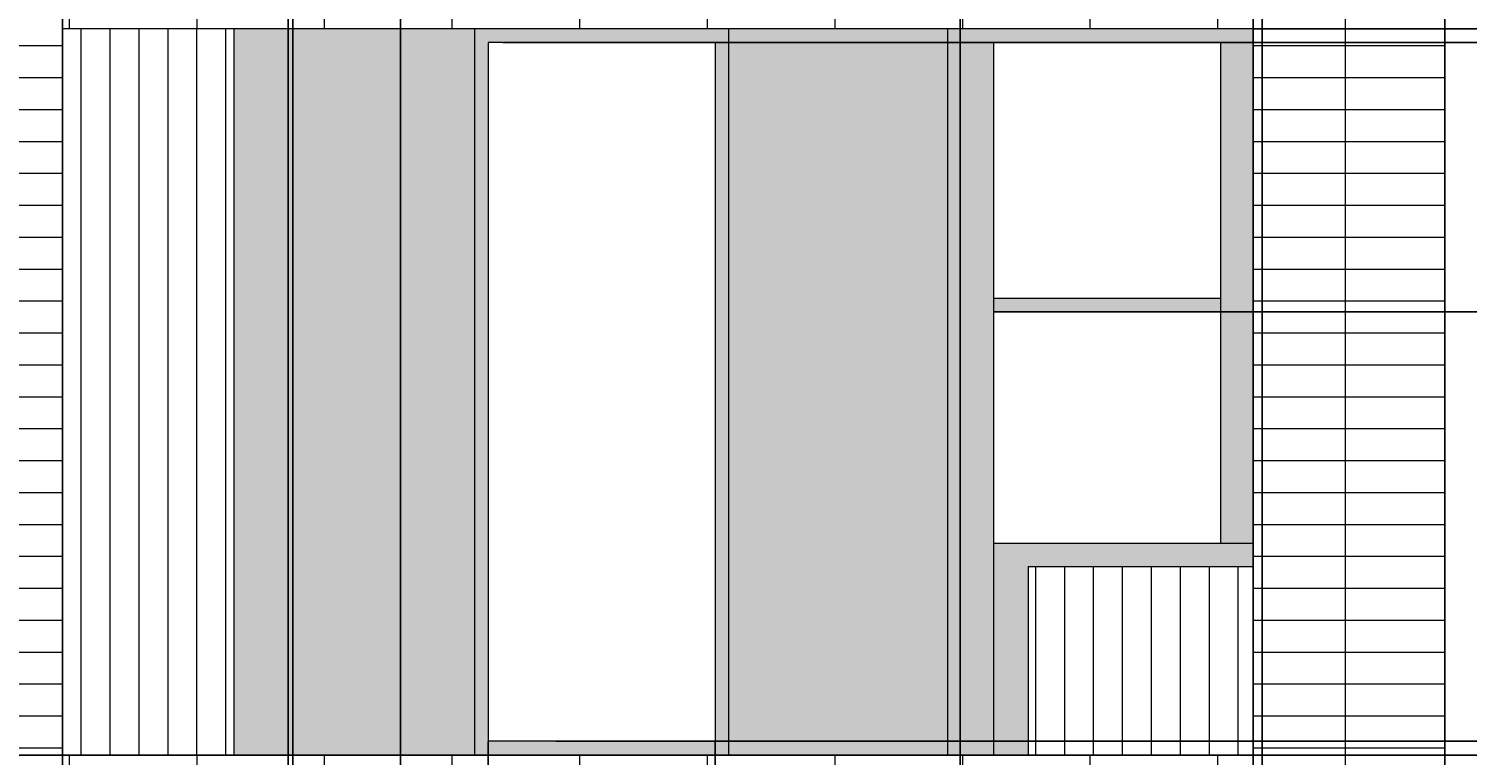
# Model space of a CAD drawing. Units: inches. Extents: x 241 to 943, y 109 to 1396.
# Tile 16 of 34: x 613 to 824, y 735 to 842. Entities that reach past the tile are written whole.
import ezdxf

# ---------------------------------------------------------------- set-up
doc = ezdxf.new("R2010")
doc.units = ezdxf.units.IN
doc.header["$MEASUREMENT"] = 0
for name, color, linetype, lineweight in [('A-ANNO-DIMS', 2, 'Continuous', 18), ('A-ELEV', 7, 'Continuous', 25), ('A-ELEV-SHAD', 9, 'Continuous', 13), ('A-GLAZ', 4, 'Continuous', 18), ('A-GLAZ-PATT', 18, 'Continuous', 13), ('A-WALL-PATT', 8, 'Continuous', 13)]:
    doc.layers.add(name, color=color, linetype=linetype, lineweight=lineweight)
doc.styles.get("Standard").update_dxf_attribs({"font": 'arial.ttf'})
doc.dimstyles.get("Standard").update_dxf_attribs({"dimtxt": 1.4375, "dimasz": 0.18, "dimexe": 0.18, "dimexo": 0.0625, "dimgap": 0.09, "dimtad": 0, "dimtih": 1, "dimtoh": 1, "dimdec": 4, "dimzin": 0, "dimdsep": 46, "dimlunit": 4, "dimtxsty": 'Standard', "dimcen": 0.09, "dimadec": 0, "dimazin": 0, "dimtfac": 1, "dimtdec": 4, "dimtofl": 0, "dimtmove": 0, "dimatfit": 3, "dimfxl": 1, "dimtolj": 1, "dimtzin": 0, "dimarcsym": 0})

# ---------------------------------------------------------------- blocks, each defined once
blk = doc.blocks.new('*D6')
at = {"layer": 'A-ANNO-DIMS', "color": 0, "lineweight": -2, "transparency": 16777216}
for p, q in [((820.84, 232.89), (820.84, 1395.05)), ((881.67, 232.89), (881.67, 1395.05)), ((821.02, 1394.87), (848.73, 1394.87)), ((881.49, 1394.87), (853.77, 1394.87))]:
    blk.add_line(p, q, dxfattribs=at)
at = {"layer": 'A-ANNO-DIMS', "color": 0, "transparency": 16777216}
for points in [[(821.02, 1394.9), (821.02, 1394.84), (820.84, 1394.87)], [(881.49, 1394.9), (881.49, 1394.84), (881.67, 1394.87)]]:
    blk.add_solid(points, dxfattribs=at)
at = {"layer": 'Defpoints', "color": 0, "transparency": 16777216}
for p in [(881.67, 1394.87), (820.84, 232.83), (881.67, 232.83)]:
    blk.add_point(p, dxfattribs=at)
at = {"layer": 'A-ANNO-DIMS', "color": 0, "transparency": 16777216, "insert": (851.25, 1394.87), "char_height": 1.438, "attachment_point": 5}
blk.add_mtext('\\A1;60.83', dxfattribs=at)
blk = doc.blocks.new('*D12')
at = {"layer": 'A-ANNO-DIMS', "color": 0, "lineweight": -2, "transparency": 16777216}
for p, q in [((530.23, 384.24), (530.23, 1395.05)), ((650.91, 384.24), (650.91, 1395.05)), ((530.41, 1394.87), (587.56, 1394.87)), ((650.73, 1394.87), (593.58, 1394.87))]:
    blk.add_line(p, q, dxfattribs=at)
at = {"layer": 'A-ANNO-DIMS', "color": 0, "transparency": 16777216}
for points in [[(530.41, 1394.9), (530.41, 1394.84), (530.23, 1394.87)], [(650.73, 1394.9), (650.73, 1394.84), (650.91, 1394.87)]]:
    blk.add_solid(points, dxfattribs=at)
at = {"layer": 'Defpoints', "color": 0, "transparency": 16777216}
for p in [(650.91, 1394.87), (530.23, 384.18), (650.91, 384.18)]:
    blk.add_point(p, dxfattribs=at)
at = {"layer": 'A-ANNO-DIMS', "color": 0, "transparency": 16777216, "insert": (590.57, 1394.87), "char_height": 1.438, "attachment_point": 5}
blk.add_mtext('\\A1;120.68', dxfattribs=at)
blk = doc.blocks.new('*D13')
at = {"layer": 'A-ANNO-DIMS', "color": 0, "lineweight": -2, "transparency": 16777216}
for p, q in [((650.91, 384.24), (650.91, 1395.05)), ((667.39, 290.06), (667.39, 1395.05)), ((651.09, 1394.87), (656.14, 1394.87)), ((667.21, 1394.87), (662.16, 1394.87))]:
    blk.add_line(p, q, dxfattribs=at)
at = {"layer": 'A-ANNO-DIMS', "color": 0, "transparency": 16777216}
for points in [[(651.09, 1394.9), (651.09, 1394.84), (650.91, 1394.87)], [(667.21, 1394.9), (667.21, 1394.84), (667.39, 1394.87)]]:
    blk.add_solid(points, dxfattribs=at)
at = {"layer": 'Defpoints', "color": 0, "transparency": 16777216}
for p in [(667.39, 1394.87), (650.91, 384.18), (667.39, 290)]:
    blk.add_point(p, dxfattribs=at)
at = {"layer": 'A-ANNO-DIMS', "color": 0, "transparency": 16777216, "insert": (659.15, 1394.87), "char_height": 1.438, "attachment_point": 5}
blk.add_mtext('\\A1;16.486', dxfattribs=at)
blk = doc.blocks.new('*D14')
at = {"layer": 'A-ANNO-DIMS', "color": 0, "lineweight": -2, "transparency": 16777216}
for p, q in [((667.39, 290.06), (667.39, 1395.05)), ((794.03, 290.06), (794.03, 1395.05)), ((667.57, 1394.87), (727.7, 1394.87)), ((793.85, 1394.87), (733.72, 1394.87))]:
    blk.add_line(p, q, dxfattribs=at)
at = {"layer": 'A-ANNO-DIMS', "color": 0, "transparency": 16777216}
for points in [[(667.57, 1394.9), (667.57, 1394.84), (667.39, 1394.87)], [(793.85, 1394.9), (793.85, 1394.84), (794.03, 1394.87)]]:
    blk.add_solid(points, dxfattribs=at)
at = {"layer": 'Defpoints', "color": 0, "transparency": 16777216}
for p in [(794.03, 1394.87), (667.39, 290), (794.03, 290)]:
    blk.add_point(p, dxfattribs=at)
at = {"layer": 'A-ANNO-DIMS', "color": 0, "transparency": 16777216, "insert": (730.71, 1394.87), "char_height": 1.438, "attachment_point": 5}
blk.add_mtext('\\A1;126.63', dxfattribs=at)
blk = doc.blocks.new('*D15')
at = {"layer": 'A-ANNO-DIMS', "color": 0, "lineweight": -2, "transparency": 16777216}
for p, q in [((794.03, 290.06), (794.03, 1395.05)), ((820.84, 232.89), (820.84, 1395.05)), ((794.21, 1394.87), (805.04, 1394.87)), ((820.66, 1394.87), (809.82, 1394.87))]:
    blk.add_line(p, q, dxfattribs=at)
at = {"layer": 'A-ANNO-DIMS', "color": 0, "transparency": 16777216}
for points in [[(794.21, 1394.9), (794.21, 1394.84), (794.03, 1394.87)], [(820.66, 1394.9), (820.66, 1394.84), (820.84, 1394.87)]]:
    blk.add_solid(points, dxfattribs=at)
at = {"layer": 'Defpoints', "color": 0, "transparency": 16777216}
for p in [(820.84, 1394.87), (794.03, 290), (820.84, 232.83)]:
    blk.add_point(p, dxfattribs=at)
at = {"layer": 'A-ANNO-DIMS', "color": 0, "transparency": 16777216, "insert": (807.43, 1394.87), "char_height": 1.438, "attachment_point": 5}
blk.add_mtext('\\A1;26.81', dxfattribs=at)
blk = doc.blocks.new('*D47')
at = {"layer": 'A-ANNO-DIMS', "color": 0, "lineweight": -2, "transparency": 16777216}
for p, q in [((792.75, 841.54), (940.6, 841.54)), ((940.42, 841.36), (940.42, 789.02)), ((940.42, 735.03), (940.42, 787.37)), ((792.75, 734.85), (940.6, 734.85))]:
    blk.add_line(p, q, dxfattribs=at)
at = {"layer": 'A-ANNO-DIMS', "color": 0, "transparency": 16777216}
for points in [[(940.39, 841.36), (940.45, 841.36), (940.42, 841.54)], [(940.39, 735.03), (940.45, 735.03), (940.42, 734.85)]]:
    blk.add_solid(points, dxfattribs=at)
at = {"layer": 'Defpoints', "color": 0, "transparency": 16777216}
for p in [(792.69, 841.54), (940.42, 841.54), (792.69, 734.85)]:
    blk.add_point(p, dxfattribs=at)
at = {"layer": 'A-ANNO-DIMS', "color": 0, "transparency": 16777216, "insert": (940.42, 788.2), "char_height": 1.438, "attachment_point": 5}
blk.add_mtext('\\A1;106.68', dxfattribs=at)
blk = doc.blocks.new('*D63')
at = {"layer": 'A-ANNO-DIMS', "color": 0, "lineweight": -2, "transparency": 16777216}
for p, q in [((651.6, 568.89), (651.6, 1395.05)), ((792.69, 568.89), (792.69, 1395.05)), ((651.78, 1394.87), (719.84, 1394.87)), ((792.51, 1394.87), (724.45, 1394.87))]:
    blk.add_line(p, q, dxfattribs=at)
at = {"layer": 'A-ANNO-DIMS', "color": 0, "transparency": 16777216}
for points in [[(651.78, 1394.9), (651.78, 1394.84), (651.6, 1394.87)], [(792.51, 1394.9), (792.51, 1394.84), (792.69, 1394.87)]]:
    blk.add_solid(points, dxfattribs=at)
at = {"layer": 'Defpoints', "color": 0, "transparency": 16777216}
for p in [(792.69, 1394.87), (651.6, 568.83), (792.69, 568.83)]:
    blk.add_point(p, dxfattribs=at)
at = {"layer": 'A-ANNO-DIMS', "color": 0, "transparency": 16777216, "insert": (722.14, 1394.87), "char_height": 1.438, "attachment_point": 5}
blk.add_mtext('\\A1;141.1', dxfattribs=at)
blk = doc.blocks.new('*D64')
at = {"layer": 'A-ANNO-DIMS', "color": 0, "lineweight": -2, "transparency": 16777216}
for p, q in [((792.69, 568.89), (792.69, 1395.05)), ((820.84, 568.89), (820.84, 1395.05)), ((792.87, 1394.87), (803.68, 1394.87)), ((820.66, 1394.87), (809.85, 1394.87))]:
    blk.add_line(p, q, dxfattribs=at)
at = {"layer": 'A-ANNO-DIMS', "color": 0, "transparency": 16777216}
for points in [[(792.87, 1394.9), (792.87, 1394.84), (792.69, 1394.87)], [(820.66, 1394.9), (820.66, 1394.84), (820.84, 1394.87)]]:
    blk.add_solid(points, dxfattribs=at)
at = {"layer": 'Defpoints', "color": 0, "transparency": 16777216}
for p in [(820.84, 1394.87), (792.69, 568.83), (820.84, 568.83)]:
    blk.add_point(p, dxfattribs=at)
at = {"layer": 'A-ANNO-DIMS', "color": 0, "transparency": 16777216, "insert": (806.76, 1394.87), "char_height": 1.438, "attachment_point": 5}
blk.add_mtext('\\A1;28.146', dxfattribs=at)
blk = doc.blocks.new('*D66')
at = {"layer": 'A-ANNO-DIMS', "color": 0, "lineweight": -2, "transparency": 16777216}
for p, q in [((617.76, 702.85), (617.76, 1395.05)), ((749.63, 702.85), (749.63, 1395.05)), ((617.94, 1394.87), (680.69, 1394.87)), ((749.45, 1394.87), (686.7, 1394.87))]:
    blk.add_line(p, q, dxfattribs=at)
at = {"layer": 'A-ANNO-DIMS', "color": 0, "transparency": 16777216}
for points in [[(617.94, 1394.9), (617.94, 1394.84), (617.76, 1394.87)], [(749.45, 1394.9), (749.45, 1394.84), (749.63, 1394.87)]]:
    blk.add_solid(points, dxfattribs=at)
at = {"layer": 'Defpoints', "color": 0, "transparency": 16777216}
for p in [(749.63, 1394.87), (617.76, 702.79), (749.63, 702.79)]:
    blk.add_point(p, dxfattribs=at)
at = {"layer": 'A-ANNO-DIMS', "color": 0, "transparency": 16777216, "insert": (683.7, 1394.87), "char_height": 1.438, "attachment_point": 5}
blk.add_mtext('\\A1;131.87', dxfattribs=at)
blk = doc.blocks.new('*D82')
at = {"layer": 'A-ANNO-DIMS', "color": 0, "lineweight": -2, "transparency": 16777216}
for p, q in [((565.2, 568.89), (565.2, 1395.05)), ((651.6, 568.89), (651.6, 1395.05)), ((565.38, 1394.87), (605.89, 1394.87)), ((651.42, 1394.87), (610.91, 1394.87))]:
    blk.add_line(p, q, dxfattribs=at)
at = {"layer": 'A-ANNO-DIMS', "color": 0, "transparency": 16777216}
for points in [[(565.38, 1394.9), (565.38, 1394.84), (565.2, 1394.87)], [(651.42, 1394.9), (651.42, 1394.84), (651.6, 1394.87)]]:
    blk.add_solid(points, dxfattribs=at)
at = {"layer": 'Defpoints', "color": 0, "transparency": 16777216}
for p in [(651.6, 1394.87), (565.2, 568.83), (651.6, 568.83)]:
    blk.add_point(p, dxfattribs=at)
at = {"layer": 'A-ANNO-DIMS', "color": 0, "transparency": 16777216, "insert": (608.4, 1394.87), "char_height": 1.438, "attachment_point": 5}
blk.add_mtext('\\A1;86.40', dxfattribs=at)
blk = doc.blocks.new('*D83')
at = {"layer": 'A-ANNO-DIMS', "color": 0, "lineweight": -2, "transparency": 16777216}
for p, q in [((592.95, 700.85), (592.95, 1395.05)), ((617.76, 702.85), (617.76, 1395.05)), ((593.13, 1394.87), (602.27, 1394.87)), ((617.58, 1394.87), (608.45, 1394.87))]:
    blk.add_line(p, q, dxfattribs=at)
at = {"layer": 'A-ANNO-DIMS', "color": 0, "transparency": 16777216}
for points in [[(593.13, 1394.9), (593.13, 1394.84), (592.95, 1394.87)], [(617.58, 1394.9), (617.58, 1394.84), (617.76, 1394.87)]]:
    blk.add_solid(points, dxfattribs=at)
at = {"layer": 'Defpoints', "color": 0, "transparency": 16777216}
for p in [(617.76, 1394.87), (617.76, 702.79), (592.95, 700.79)]:
    blk.add_point(p, dxfattribs=at)
at = {"layer": 'A-ANNO-DIMS', "color": 0, "transparency": 16777216, "insert": (605.36, 1394.87), "char_height": 1.438, "attachment_point": 5}
blk.add_mtext('\\A1;24.805', dxfattribs=at)
blk = doc.blocks.new('*D84')
at = {"layer": 'A-ANNO-DIMS', "color": 0, "lineweight": -2, "transparency": 16777216}
for p, q in [((749.63, 702.85), (749.63, 1395.05)), ((820.84, 736.89), (820.84, 1395.05)), ((749.81, 1394.87), (782.73, 1394.87)), ((820.66, 1394.87), (787.74, 1394.87))]:
    blk.add_line(p, q, dxfattribs=at)
at = {"layer": 'A-ANNO-DIMS', "color": 0, "transparency": 16777216}
for points in [[(749.81, 1394.9), (749.81, 1394.84), (749.63, 1394.87)], [(820.66, 1394.9), (820.66, 1394.84), (820.84, 1394.87)]]:
    blk.add_solid(points, dxfattribs=at)
at = {"layer": 'Defpoints', "color": 0, "transparency": 16777216}
for p in [(820.84, 1394.87), (820.84, 736.83), (749.63, 702.79)]:
    blk.add_point(p, dxfattribs=at)
at = {"layer": 'A-ANNO-DIMS', "color": 0, "transparency": 16777216, "insert": (785.24, 1394.87), "char_height": 1.438, "attachment_point": 5}
blk.add_mtext('\\A1;71.20', dxfattribs=at)
blk = doc.blocks.new('*D99')
at = {"layer": 'A-ANNO-DIMS', "color": 0, "lineweight": -2, "transparency": 16777216}
for p, q in [((417.09, 181.71), (417.09, 1395.05)), ((667.39, 214.58), (667.39, 1395.05)), ((417.27, 1394.87), (539.16, 1394.87)), ((667.21, 1394.87), (545.33, 1394.87))]:
    blk.add_line(p, q, dxfattribs=at)
at = {"layer": 'A-ANNO-DIMS', "color": 0, "transparency": 16777216}
for points in [[(417.27, 1394.9), (417.27, 1394.84), (417.09, 1394.87)], [(667.21, 1394.9), (667.21, 1394.84), (667.39, 1394.87)]]:
    blk.add_solid(points, dxfattribs=at)
at = {"layer": 'Defpoints', "color": 0, "transparency": 16777216}
for p in [(667.39, 1394.87), (667.39, 214.52), (417.09, 181.65)]:
    blk.add_point(p, dxfattribs=at)
at = {"layer": 'A-ANNO-DIMS', "color": 0, "transparency": 16777216, "insert": (542.24, 1394.87), "char_height": 1.438, "attachment_point": 5}
blk.add_mtext('\\A1;250.30', dxfattribs=at)
blk = doc.blocks.new('*D121')
at = {"layer": 'A-ANNO-DIMS', "color": 0, "lineweight": -2, "transparency": 16777216}
for p, q in [((680.27, 736.86), (680.27, 109.81)), ((713.62, 736.86), (713.62, 109.81)), ((680.45, 109.99), (693.87, 109.99)), ((713.44, 109.99), (700.02, 109.99))]:
    blk.add_line(p, q, dxfattribs=at)
at = {"layer": 'A-ANNO-DIMS', "color": 0, "transparency": 16777216}
for points in [[(680.45, 110.02), (680.45, 109.96), (680.27, 109.99)], [(713.44, 110.02), (713.44, 109.96), (713.62, 109.99)]]:
    blk.add_solid(points, dxfattribs=at)
at = {"layer": 'Defpoints', "color": 0, "transparency": 16777216}
for p in [(680.27, 736.92), (713.62, 736.92), (713.62, 109.99)]:
    blk.add_point(p, dxfattribs=at)
at = {"layer": 'A-ANNO-DIMS', "color": 0, "transparency": 16777216, "insert": (696.95, 109.99), "char_height": 1.438, "attachment_point": 5}
blk.add_mtext('\\A1;33.356', dxfattribs=at)
blk = doc.blocks.new('*D124')
at = {"layer": 'A-ANNO-DIMS', "color": 0, "lineweight": -2, "transparency": 16777216}
for p, q in [((682.52, 839.54), (940.6, 839.54)), ((940.42, 839.36), (940.42, 789.05)), ((940.42, 737.1), (940.42, 787.41)), ((690.27, 736.92), (940.6, 736.92))]:
    blk.add_line(p, q, dxfattribs=at)
at = {"layer": 'A-ANNO-DIMS', "color": 0, "transparency": 16777216}
for points in [[(940.39, 839.36), (940.45, 839.36), (940.42, 839.54)], [(940.39, 737.1), (940.45, 737.1), (940.42, 736.92)]]:
    blk.add_solid(points, dxfattribs=at)
at = {"layer": 'Defpoints', "color": 0, "transparency": 16777216}
for p in [(682.45, 839.54), (940.42, 839.54), (690.2, 736.92)]:
    blk.add_point(p, dxfattribs=at)
at = {"layer": 'A-ANNO-DIMS', "color": 0, "transparency": 16777216, "insert": (940.42, 788.23), "char_height": 1.438, "attachment_point": 5}
blk.add_mtext('\\A1;102.61', dxfattribs=at)
blk = doc.blocks.new('*D125')
at = {"layer": 'A-ANNO-DIMS', "color": 0, "lineweight": -2, "transparency": 16777216}
for p, q in [((754.6, 799.98), (940.6, 799.98)), ((940.42, 799.8), (940.42, 768.24)), ((940.42, 735.03), (940.42, 766.59)), ((759.69, 734.85), (940.6, 734.85))]:
    blk.add_line(p, q, dxfattribs=at)
at = {"layer": 'A-ANNO-DIMS', "color": 0, "transparency": 16777216}
for points in [[(940.39, 799.8), (940.45, 799.8), (940.42, 799.98)], [(940.39, 735.03), (940.45, 735.03), (940.42, 734.85)]]:
    blk.add_solid(points, dxfattribs=at)
at = {"layer": 'Defpoints', "color": 0, "transparency": 16777216}
for p in [(754.54, 799.98), (940.42, 799.98), (759.62, 734.85)]:
    blk.add_point(p, dxfattribs=at)
at = {"layer": 'A-ANNO-DIMS', "color": 0, "transparency": 16777216, "insert": (940.42, 767.42), "char_height": 1.438, "attachment_point": 5}
blk.add_mtext('\\A1;65.13', dxfattribs=at)

msp = doc.modelspace()

# ---------------------------------------------------------------- hatches: boundary and pattern name
at = {"layer": 'A-ELEV-SHAD'}
h = msp.add_hatch(color=256, dxfattribs=at)
h.dxf.hatch_style = 1
h.paths.add_polyline_path([(537.4269, 698.7912), (534.1778, 698.7912), (534.1778, 659.3434), (537.4269, 659.3434)])
h.paths.add_polyline_path([(508.0803, 698.7912), (450.9259, 698.7912), (450.9259, 659.3434), (452.9259, 659.3434), (452.9259, 696.7912), (506.0803, 696.7912), (506.0803, 659.3434), (508.0803, 659.3434)])
h.paths.add_polyline_path([(481.5031, 696.7912), (479.5031, 696.7912), (479.5031, 659.3434), (481.5031, 659.3434)], flags=17)
h.paths.add_polyline_path([(481.5031, 657.3434), (479.5031, 657.3434), (479.5031, 653.3371), (481.5031, 653.3371)], flags=17)
h.paths.add_polyline_path([(508.0803, 657.3434), (506.0803, 657.3434), (506.0803, 653.3371), (452.9259, 653.3371), (452.9259, 657.3434), (450.9259, 657.3434), (450.9259, 651.3371), (508.0803, 651.3371)])
h.paths.add_polyline_path([(428.1173, 839.5382), (426.1173, 839.5382), (426.1173, 786.9154), (428.1173, 786.9154)], flags=17)
h.paths.add_polyline_path([(470.8692, 839.5382), (468.8692, 839.5382), (468.8692, 786.9154), (470.8692, 786.9154)], flags=17)
h.paths.add_polyline_path([(508.3064, 841.5382), (396.3125, 841.5382), (396.3125, 782.5808), (398.3125, 782.5808), (398.3125, 839.5382), (506.3064, 839.5382), (506.3064, 782.5808), (508.3064, 782.5808)])
h.paths.add_polyline_path([(398.3125, 780.5808), (396.3125, 780.5808), (396.3125, 773.4916), (398.3125, 773.4916)])
h.paths.add_polyline_path([(508.3064, 780.5808), (506.3064, 780.5808), (506.3064, 773.4916), (508.3064, 773.4916)])
h.paths.add_polyline_path([(715.6236, 841.5382), (678.2674, 841.5382), (678.2674, 734.8538), (715.6236, 734.8538)])
h.paths.add_polyline_path([(680.2674, 839.5382), (682.4526, 839.5382), (713.6236, 839.5382), (713.6236, 736.9235), (690.2047, 736.9235), (680.2674, 736.9235)], flags=16)
h.paths.add_polyline_path([(792.691, 841.5382), (747.7579, 841.5382), (747.7579, 734.8538), (754.5373, 734.8538), (754.5373, 736.9235), (754.5373, 839.5382), (756.7224, 839.5382), (787.8934, 839.5382), (787.8934, 765.9585), (792.691, 765.9585)])
h.paths.add_polyline_path([(659.2925, 1009.5382), (657.2925, 1009.5382), (657.2925, 902.8538), (659.2925, 902.8538)])
h.paths.add_polyline_path([(751.5078, 976.6275), (712.5839, 976.6275), (712.5839, 974.6275), (751.5078, 974.6275)])
h.paths.add_polyline_path([(470.8692, 1007.5382), (468.8692, 1007.5382), (468.8692, 954.9154), (470.8692, 954.9154)], flags=17)
h.paths.add_polyline_path([(508.3064, 1009.5382), (396.3125, 1009.5382), (396.3125, 950.5808), (398.3125, 950.5808), (398.3125, 1007.5382), (506.3064, 1007.5382), (506.3064, 950.5808), (508.3064, 950.5808)])
h.paths.add_polyline_path([(428.1173, 1007.5382), (426.1173, 1007.5382), (426.1173, 954.9154), (428.1173, 954.9154)], flags=17)
h.paths.add_polyline_path([(398.3125, 948.5808), (396.3125, 948.5808), (396.3125, 941.4916), (398.3125, 941.4916)])
h.paths.add_polyline_path([(508.3064, 948.5808), (506.3064, 948.5808), (506.3064, 941.4916), (508.3064, 941.4916)])
h.paths.add_polyline_path([(428.1173, 1175.5382), (426.1173, 1175.5382), (426.1173, 1122.9154), (428.1173, 1122.9154)], flags=17)
h.paths.add_polyline_path([(508.3064, 1177.5382), (396.3125, 1177.5382), (396.3125, 1118.5808), (398.3125, 1118.5808), (398.3125, 1175.5382), (506.3064, 1175.5382), (506.3064, 1118.5808), (506.8039, 1118.5808, -1), (506.8039, 1116.5808), (506.3064, 1116.5808), (506.3064, 1109.4916), (508.3064, 1109.4916)])
h.paths.add_polyline_path([(470.8692, 1175.5382), (468.8692, 1175.5382), (468.8692, 1122.9154), (470.8692, 1122.9154)], flags=17)
h.paths.add_polyline_path([(398.3125, 1116.5808), (396.3125, 1116.5808), (396.3125, 1109.4916), (398.3125, 1109.4916)], flags=17)
h.paths.add_polyline_path([(724.819, 1177.7336), (533.952, 1177.7336), (533.952, 1108.1686), (724.819, 1108.1686)])
h.paths.add_polyline_path([(535.952, 1175.7336), (722.819, 1175.7336), (722.819, 1110.1686), (535.952, 1110.1686)], flags=0)
h.paths.add_polyline_path([(622.521, 1136.0739), (643.4534, 1136.0739), (643.4534, 1134.0739), (622.521, 1134.0739)], flags=0)
h.paths.add_polyline_path([(722.819, 1175.7336), (535.952, 1175.7336), (535.952, 1110.1686), (722.819, 1110.1686)], flags=16)
h.paths.add_polyline_path([(565.947, 1151.5772), (535.952, 1151.5772), (535.952, 1149.5772), (565.947, 1149.5772)], flags=0)
h = msp.add_hatch(color=256, dxfattribs=at)
h.dxf.hatch_style = 1
h.paths.add_polyline_path([(537.4269, 657.3434), (534.1778, 657.3434), (534.1778, 651.3371), (537.4269, 651.3371)])
h.paths.add_polyline_path([(563.9297, 657.3434), (563.2023, 657.3434), (563.2023, 651.3371), (563.9297, 651.3371)])
h.paths.add_polyline_path([(563.9297, 698.7912), (563.2023, 698.7912), (563.2023, 659.3434), (563.9297, 659.3434)])
h.paths.add_polyline_path([(787.8934, 801.9791), (754.5373, 801.9791), (754.5373, 799.9791), (787.8934, 799.9791)])
h = msp.add_hatch(color=256, dxfattribs=at)
h.dxf.hatch_style = 1
h.paths.add_polyline_path([(759.6248, 762.5799), (792.691, 762.5799), (792.691, 765.9585), (754.5373, 765.9585), (754.5373, 736.9235), (754.5373, 734.8538), (759.6248, 734.8538), (759.6248, 736.9235)])
h.paths.add_polyline_path([(446.4348, 651.3371), (428.0291, 651.3371), (428.0291, 698.7912), (426.1086, 698.7912), (426.1086, 643.7483), (446.4348, 643.7483)])
at = {"layer": 'A-GLAZ-PATT'}
h = msp.add_hatch(dxfattribs=at)
h.set_pattern_fill('GOST_GLASS', color=256, scale=0.89)
h.set_pattern_definition([(45, (0, 0), (7.5519, 0), [4.45, -6.23]), (45, (1.888, 0), (7.5519, 0), [1.78, -8.9]), (45, (0, 1.888), (7.5519, 0), [1.78, -8.9])])
h.paths.add_polyline_path([(676.8698, 700.7912), (652.0129, 700.7912), (652.0129, 628.4013), (676.8698, 628.4013)])
h.paths.add_polyline_path([(650.0129, 700.7912), (617.7594, 700.7912), (617.7594, 628.4013), (650.0129, 628.4013)])
h.paths.add_polyline_path([(747.7579, 841.5382), (715.6236, 841.5382), (715.6236, 734.8538), (747.7579, 734.8538)])
h.paths.add_polyline_path([(678.2674, 841.5382), (642.9197, 841.5382), (642.9197, 734.8538), (678.2674, 734.8538)])
h.paths.add_polyline_path([(712.5839, 1009.5382), (677.6886, 1009.5382), (677.6886, 902.8538), (712.5839, 902.8538)])
h.paths.add_polyline_path([(640.1141, 1009.5382), (603.8694, 1009.5382), (603.8694, 902.8538), (640.1141, 902.8538)])
h.paths.add_polyline_path([(682.8748, 1175.7336), (643.4534, 1175.7336), (643.4534, 1110.1686), (682.8748, 1110.1686)])
h.paths.add_polyline_path([(602.3616, 1175.7336), (565.947, 1175.7336), (565.947, 1110.1686), (602.3616, 1110.1686)])
h = msp.add_hatch(dxfattribs=at)
h.set_pattern_fill('ANSI31', color=256, scale=34, angle=45)
h.paths.add_polyline_path([(722.819, 1175.7336), (682.8748, 1175.7336), (682.8748, 1110.1686), (722.819, 1110.1686)])
h.paths.add_polyline_path([(642.9197, 841.5382), (617.7594, 841.5382), (617.7594, 734.8538), (642.9197, 734.8538)])
h = msp.add_hatch(dxfattribs=at)
h.set_pattern_fill('ANSI31', color=256, scale=34, angle=45)
h.paths.add_polyline_path([(486.3418, 786.9154), (413.1187, 786.9154), (413.1187, 761.2284), (486.3418, 761.2284)])
h.paths.add_polyline_path([(486.3418, 954.9154), (413.1187, 954.9154), (413.1187, 929.2284), (486.3418, 929.2284)])
h.paths.add_polyline_path([(462.1074, 289.6933), (390.895, 289.6933), (390.895, 277.4626), (390.895, 274.3507), (462.1074, 274.3507), (462.1074, 277.4626)])
h.paths.add_polyline_path([(500.3323, 289.6933), (479.596, 289.6933), (479.596, 274.3507), (500.3323, 274.3507)])
h.paths.add_polyline_path([(450.9259, 566.8295), (426.1086, 566.8295), (426.1086, 498.4395), (446.4348, 498.4395), (446.4348, 519.3754), (450.9259, 519.3754), (450.9259, 525.3816), (445.5808, 525.3816, -1), (445.5808, 527.3816), (450.9259, 527.3816)])
h.paths.add_polyline_path([(563.2023, 508.9074), (534.1778, 508.9074), (508.1906, 508.9074), (508.1906, 498.4395), (563.2023, 498.4395)])
h.paths.add_polyline_path([(747.6328, 700.7912), (712.0171, 700.7912), (712.0171, 628.4013), (747.6328, 628.4013)])
h.paths.add_polyline_path([(446.4348, 643.7483), (426.1086, 643.7483), (426.1086, 630.4013), (446.4348, 630.4013)])
h.paths.add_polyline_path([(564.8076, 841.5382), (553.5166, 841.5382), (508.3064, 841.5382), (508.3064, 782.5808), (564.8076, 782.5808)])
h.paths.add_polyline_path([(564.8076, 780.5808), (508.3064, 780.5808), (508.3064, 773.4916), (564.8076, 773.4916)])
h.paths.add_polyline_path([(792.691, 762.5799), (759.6248, 762.5799), (759.6248, 736.9235), (759.6248, 734.8538), (792.691, 734.8538)])
h.paths.add_polyline_path([(564.8076, 1009.5382), (553.5166, 1009.5382), (508.3064, 1009.5382), (508.3064, 950.5808), (562.3033, 950.5808, -1), (562.3033, 948.5808), (508.3064, 948.5808), (508.3064, 941.4916), (564.8076, 941.4916)])
h.paths.add_polyline_path([(486.3418, 1122.9154), (413.1187, 1122.9154), (413.1187, 1097.2284), (486.3418, 1097.2284)])
at = {"layer": 'A-WALL-PATT'}
h = msp.add_hatch(dxfattribs=at)
h.set_pattern_fill('GRATE', color=256, scale=150)
h.paths.add_polyline_path([(747.7579, 1238.8538), (747.7579, 1275.9142), (747.7579, 1336.1154), (508.3064, 1336.1154), (508.3064, 1275.9142), (508.3064, 1238.8538), (508.3064, 1177.5382), (508.3064, 1109.4916), (508.3064, 1070.8538), (553.5166, 1070.8538), (749.6328, 1070.8538)])
h.paths.add_polyline_path([(533.952, 1108.1686), (533.952, 1177.7336), (533.952, 1303.0286), (724.819, 1303.0286), (724.819, 1108.1686)], flags=16)
h.paths.add_polyline_path([(535.952, 1110.1686), (535.952, 1175.7336), (722.819, 1175.7336), (722.819, 1110.1686)], flags=0)
h.paths.add_polyline_path([(643.4534, 1134.0739), (622.521, 1134.0739), (622.521, 1136.0739), (643.4534, 1136.0739)], flags=0)
h.paths.add_polyline_path([(617.7594, 568.8295), (617.7594, 734.8538), (377.0391, 734.8538), (377.0391, 566.8538), (377.0391, 400.8295), (417.0913, 400.8295), (618.9643, 400.8295)])
h.paths.add_polyline_path([(424.1086, 496.4395), (424.1086, 568.8295), (565.2023, 568.8295), (565.2023, 496.4395)], flags=16)
h.paths.add_polyline_path([(426.1086, 498.4395), (426.1086, 566.8295), (563.2023, 566.8295), (563.2023, 508.9074), (563.2023, 498.4395)], flags=0)
h.paths.add_polyline_path([(508.0803, 508.9074), (508.0803, 519.3754), (450.9259, 519.3754), (450.9259, 525.3816), (445.5808, 525.3816, -1), (445.5808, 527.3816), (450.9259, 527.3816), (450.9259, 566.8295), (508.0803, 566.8295), (537.4269, 566.8295), (537.4269, 508.9074)], flags=0)
h.paths.add_polyline_path([(506.0803, 521.3754), (452.9259, 521.3754), (452.9259, 564.8295), (506.0803, 564.8295)], flags=0)
h.paths.add_polyline_path([(424.1086, 628.4013), (424.1086, 700.7912), (592.9542, 700.7912), (592.9542, 628.4013)], flags=16)
h.paths.add_polyline_path([(426.1086, 630.4013), (426.1086, 698.7912), (590.8792, 698.7912), (590.8792, 630.4013)], flags=0)
h.paths.add_polyline_path([(508.1906, 651.3371), (508.0803, 651.3371), (450.9259, 651.3371), (428.0291, 651.3371), (428.0291, 698.7912), (451.9767, 698.7912), (508.0803, 698.7912), (537.4269, 698.7912), (563.2023, 698.7912), (563.2023, 659.3434), (563.9297, 659.3434), (563.9297, 651.3371)], flags=0)
h.paths.add_polyline_path([(506.0803, 653.3371), (452.9259, 653.3371), (452.9259, 657.3434), (445.5808, 657.3434, -1), (445.5808, 659.3434), (452.9259, 659.3434), (452.9259, 696.7912), (506.0803, 696.7912)], flags=0)
h = msp.add_hatch(dxfattribs=at)
h.set_pattern_fill('GRATE', color=256, scale=150)
h.paths.add_polyline_path([(820.8374, 1070.8538), (749.6328, 1070.8538), (553.5166, 1070.8538), (508.3064, 1070.8538), (508.3064, 1009.5382), (553.5166, 1009.5382), (564.8076, 1009.5382), (603.8694, 1009.5382), (751.5078, 1009.5382), (751.5078, 902.8538), (603.8694, 902.8538), (603.8694, 1009.5382), (564.8076, 1009.5382), (564.8076, 941.4916), (568.1348, 941.4916), (568.1348, 902.8538), (581.3632, 902.8538), (581.3632, 841.5382), (564.8076, 841.5382), (564.8076, 782.5808), (605.9087, 782.5808, -1), (605.9087, 780.5808), (564.8076, 780.5808), (564.8076, 773.4916), (597.514, 773.4916), (607.8162, 773.4916), (607.8162, 734.8538), (617.7594, 734.8538), (617.7594, 841.5382), (792.691, 841.5382), (792.691, 734.8538), (617.7594, 734.8538), (617.7594, 702.7912), (749.6328, 702.7912), (749.6328, 626.4013), (617.7594, 626.4013), (617.7594, 568.8295), (820.8374, 568.8295), (820.8374, 736.8295), (820.8374, 902.8538)])

# ---------------------------------------------------------------- linework, layer by layer
at = {"layer": 'A-ELEV'}
for p, q in [((820.8374, 736.8295), (820.8374, 902.8538)), ((820.8374, 568.8295), (820.8374, 736.8295)), ((377.0391, 734.8538), (792.691, 734.8538)), ((617.7594, 568.8295), (617.7594, 734.8538))]:
    msp.add_line(p, q, dxfattribs=at)
at = {"layer": 'A-GLAZ'}
for p, q in [((642.9197, 841.5382), (642.9197, 734.8538)), ((678.2674, 841.5382), (678.2674, 734.8538)), ((715.6236, 841.5382), (715.6236, 734.8538)), ((747.7579, 841.5382), (747.7579, 734.8538)), ((680.2674, 839.5382), (680.2674, 736.9235)), ((682.4526, 839.5382), (680.2674, 839.5382)), ((682.4526, 839.5382), (713.6236, 839.5382)), ((713.6236, 839.5382), (713.6236, 736.9235)), ((754.5373, 839.5382), (754.5373, 736.9235)), ((756.7224, 839.5382), (754.5373, 839.5382)), ((756.7224, 839.5382), (787.8934, 839.5382)), ((787.8934, 839.5382), (787.8934, 765.9585)), ((754.5373, 801.9791), (787.8934, 801.9791)), ((754.5373, 799.9791), (787.8934, 799.9791)), ((792.691, 765.9585), (754.5373, 765.9585)), ((759.6248, 762.5799), (759.6248, 736.9235)), ((759.6248, 762.5799), (792.691, 762.5799)), ((690.2047, 736.9235), (680.2674, 736.9235)), ((690.2047, 736.9235), (713.6236, 736.9235)), ((754.5373, 736.9235), (754.5373, 734.8538)), ((759.6248, 736.9235), (759.6248, 734.8538))]:
    msp.add_line(p, q, dxfattribs=at)
msp.add_lwpolyline([(617.7594, 734.8538), (792.691, 734.8538), (792.691, 841.5382), (617.7594, 841.5382)], close=True, dxfattribs=at)

# ---------------------------------------------------------------- dimensions: what is measured, and where the dimension line sits
at = {"layer": 'A-ANNO-DIMS'}
for base, p1, p2, override, picture, middle in [((667.3935, 1394.8654), (417.0913, 181.649), (667.3935, 214.5189), {"dimdec": 2, "dimlfac": 1, "dimrnd": 0, "dimzin": 0, "dimdsep": 46, "dimlunit": 2}, '*D99', (542.2424, 1394.8654)), ((650.907, 1394.8654), (530.2303, 384.1784), (650.907, 384.1784), {"dimdec": 2, "dimlfac": 1, "dimrnd": 0, "dimzin": 0, "dimdsep": 46, "dimlunit": 2}, '*D12', (590.5686, 1394.8654)), ((651.5974, 1394.8654), (565.2023, 568.8295), (651.5974, 568.8295), {"dimdec": 2, "dimlfac": 1, "dimrnd": 0, "dimzin": 0, "dimdsep": 46, "dimlunit": 2}, '*D82', (608.3998, 1394.8654)), ((617.7594, 1394.8654), (592.9542, 700.7912), (617.7594, 702.7912), {"dimdec": 3, "dimlfac": 1, "dimrnd": 0, "dimzin": 0, "dimdsep": 46, "dimlunit": 2}, '*D83', (605.3568, 1394.8654)), ((749.6328, 1394.8654), (617.7594, 702.7912), (749.6328, 702.7912), {"dimdec": 2, "dimlfac": 1, "dimrnd": 0, "dimzin": 0, "dimdsep": 46, "dimlunit": 2}, '*D66', (683.6961, 1394.8654)), ((667.39345, 1394.86544), (650.90697, 384.17836), (667.39345, 289.99842), {"dimdec": 3, "dimlfac": 1, "dimrnd": 0, "dimzin": 0, "dimdsep": 46, "dimlunit": 2}, '*D13', (659.15021, 1394.86544)), ((792.691, 1394.8654), (651.5974, 568.8295), (792.691, 568.8295), {"dimdec": 1, "dimlfac": 1, "dimrnd": 0, "dimzin": 0, "dimdsep": 46, "dimlunit": 2}, '*D63', (722.1442, 1394.8654)), ((794.0275, 1394.8654), (667.3935, 289.9984), (794.0275, 289.9984), {"dimdec": 2, "dimlfac": 1, "dimrnd": 0, "dimzin": 0, "dimdsep": 46, "dimlunit": 2}, '*D14', (730.7105, 1394.8654)), ((820.8374, 1394.8654), (749.6328, 702.7912), (820.8374, 736.8295), {"dimdec": 2, "dimlfac": 1, "dimrnd": 0, "dimzin": 0, "dimdsep": 46, "dimlunit": 2}, '*D84', (785.2351, 1394.8654)), ((820.8374, 1394.8654), (792.691, 568.8295), (820.8374, 568.8295), {"dimdec": 3, "dimlfac": 1, "dimrnd": 0, "dimzin": 0, "dimdsep": 46, "dimlunit": 2}, '*D64', (806.7642, 1394.8654)), ((820.8374, 1394.8654), (794.0275, 289.9984), (820.8374, 232.8295), {"dimdec": 2, "dimlfac": 1, "dimrnd": 0, "dimzin": 0, "dimdsep": 46, "dimlunit": 2}, '*D15', (807.4324, 1394.8654)), ((881.667, 1394.8654), (820.8374, 232.8295), (881.667, 232.8295), {"dimdec": 2, "dimlfac": 1, "dimrnd": 0, "dimzin": 0, "dimdsep": 46, "dimlunit": 2}, '*D6', (851.2522, 1394.8654)), ((713.6236, 109.9907), (680.2674, 736.9235), (713.6236, 736.9235), {"dimdec": 3, "dimlfac": 1, "dimrnd": 0, "dimzin": 0, "dimdsep": 46, "dimlunit": 2}, '*D121', (696.9455, 109.9907))]:
    dim = msp.add_linear_dim(base=base, p1=p1, p2=p2, dimstyle='Standard', override=override, dxfattribs=at)
    dim.commit()
    dim.dimension.update_dxf_attribs({"geometry": picture, "text_midpoint": middle})
for base, p1, p2, picture, middle in [((940.417, 841.5382), (792.691, 734.8538), (792.691, 841.5382), '*D47', (940.417, 788.196)), ((940.417, 839.5382), (690.2047, 736.9235), (682.4526, 839.5382), '*D124', (940.417, 788.2308)), ((940.417, 799.9791), (759.6248, 734.8538), (754.5373, 799.9791), '*D125', (940.417, 767.4165))]:
    dim = msp.add_linear_dim(base=base, p1=p1, p2=p2, angle=90, dimstyle='Standard', override={"dimdec": 2, "dimlfac": 1, "dimrnd": 0, "dimzin": 0, "dimdsep": 46, "dimlunit": 2}, dxfattribs=at)
    dim.commit()
    dim.dimension.update_dxf_attribs({"geometry": picture, "text_midpoint": middle})

doc.saveas('drawing.dxf')
